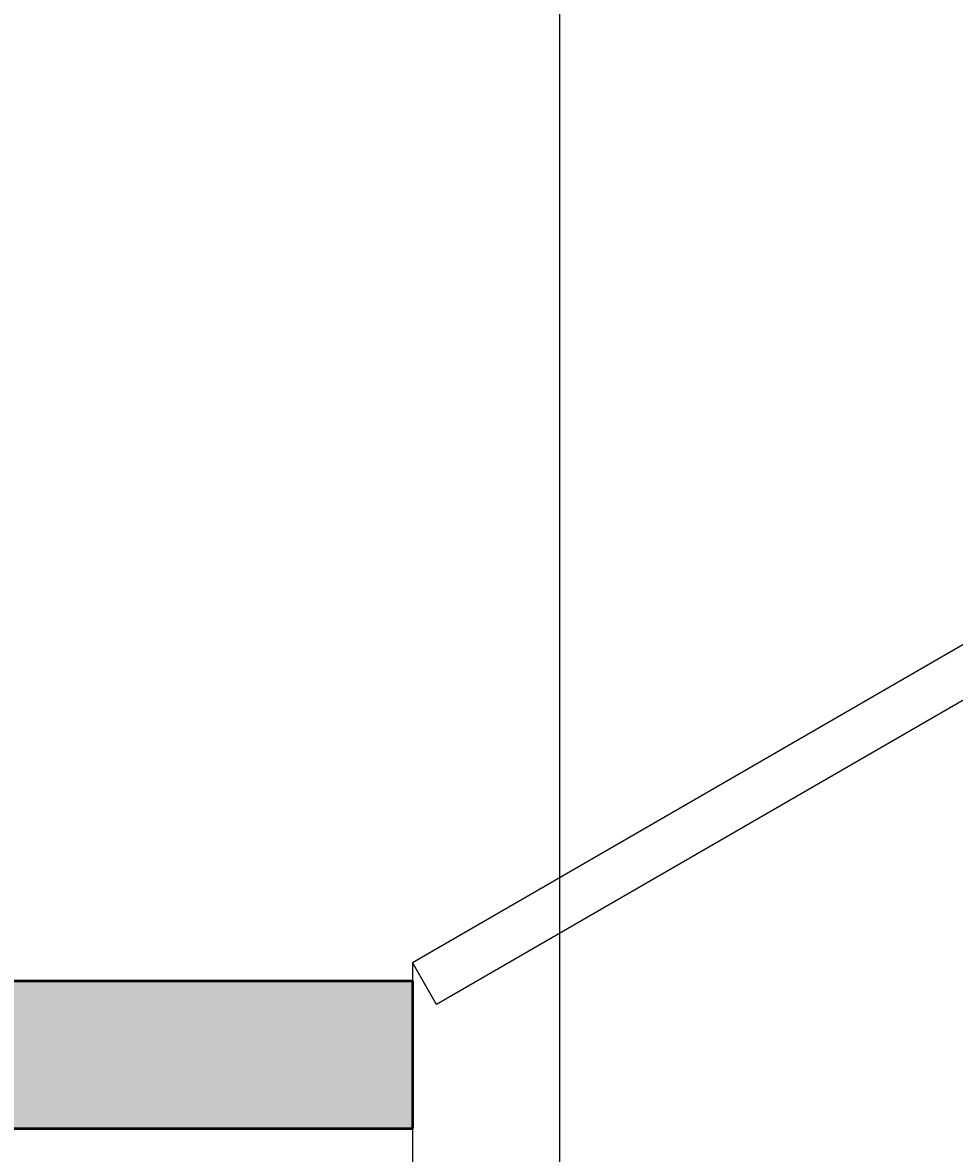
# Model space of a CAD drawing. Units: inches. Extents: x 2231 to 2461, y 2045 to 2455.
# Tile 55 of 95: x 2320 to 2346, y 2302 to 2333. Entities that reach past the tile are written whole.
import ezdxf

# ---------------------------------------------------------------- set-up
doc = ezdxf.new("R2010")
doc.units = ezdxf.units.IN
for name, color, linetype, lineweight in [('A-ANNO-DIMS', 2, 'Continuous', 18), ('A-DOOR', 3, 'Continuous', 25), ('A-WALL', 7, 'Continuous', 50)]:
    doc.layers.add(name, color=color, linetype=linetype, lineweight=lineweight)
doc.layers.add('A-WALL-PATT', color=18, linetype='Continuous', lineweight=13, true_color=0x000000)
doc.styles.get("Standard").update_dxf_attribs({"font": 'arial.ttf'})
doc.dimstyles.get("Standard").update_dxf_attribs({"dimtxt": 0.18, "dimasz": 0.18, "dimexe": 0.18, "dimexo": 0.0625, "dimgap": 0.09, "dimtad": 0, "dimtih": 1, "dimtoh": 1, "dimdec": 4, "dimzin": 0, "dimdsep": 46, "dimtxsty": 'Standard', "dimcen": 0.09, "dimadec": 0, "dimazin": 0, "dimtfac": 1, "dimtdec": 4, "dimtofl": 0, "dimtmove": 0, "dimatfit": 3, "dimfxl": 1, "dimtolj": 1, "dimtzin": 0, "dimarcsym": 0})

# ---------------------------------------------------------------- blocks, each defined once
blk = doc.blocks.new('*U3')
for p, q in [((0, 0), (0, -6)), ((40, 0), (40, -6))]:
    blk.add_line(p, q)
blk.add_lwpolyline([(0, 0), (34.641, 20), (35.516, 18.484), (0.875, -1.516)], close=True)
blk.add_arc((0, 0), 40, 0, 30)
blk = doc.blocks.new('*D50')
at = {"layer": 'A-ANNO-DIMS', "color": 0, "lineweight": -2, "transparency": 16777216}
for p, q in [((2304.794, 2182.895), (2304.794, 2454.645)), ((2304.974, 2454.465), (2319.575, 2454.465)), ((2334.614, 2454.465), (2320.012, 2454.465)), ((2334.794, 2182.895), (2334.794, 2454.645))]:
    blk.add_line(p, q, dxfattribs=at)
at = {"layer": 'A-ANNO-DIMS', "color": 0, "transparency": 16777216}
for points in [[(2304.974, 2454.495), (2304.974, 2454.435), (2304.794, 2454.465)], [(2334.614, 2454.495), (2334.614, 2454.435), (2334.794, 2454.465)]]:
    blk.add_solid(points, dxfattribs=at)
at = {"layer": 'Defpoints', "color": 0, "transparency": 16777216}
for p in [(2334.794, 2454.465), (2304.794, 2182.833), (2334.794, 2182.833)]:
    blk.add_point(p, dxfattribs=at)
at = {"layer": 'A-ANNO-DIMS', "color": 0, "transparency": 16777216, "insert": (2319.794, 2454.465), "char_height": 0.18, "attachment_point": 5}
blk.add_mtext('\\A1;30', dxfattribs=at)
blk = doc.blocks.new('*D51')
at = {"layer": 'A-ANNO-DIMS', "color": 0, "lineweight": -2, "transparency": 16777216}
for p, q in [((2258.794, 2306.77), (2258.794, 2044.803)), ((2330.794, 2306.77), (2330.794, 2044.803)), ((2258.974, 2044.983), (2294.576, 2044.983)), ((2330.614, 2044.983), (2295.011, 2044.983))]:
    blk.add_line(p, q, dxfattribs=at)
at = {"layer": 'A-ANNO-DIMS', "color": 0, "transparency": 16777216}
for points in [[(2258.974, 2045.013), (2258.974, 2044.953), (2258.794, 2044.983)], [(2330.614, 2045.013), (2330.614, 2044.953), (2330.794, 2044.983)]]:
    blk.add_solid(points, dxfattribs=at)
at = {"layer": 'Defpoints', "color": 0, "transparency": 16777216}
for p in [(2258.794, 2306.833), (2330.794, 2306.833), (2330.794, 2044.983)]:
    blk.add_point(p, dxfattribs=at)
at = {"layer": 'A-ANNO-DIMS', "color": 0, "transparency": 16777216, "insert": (2294.794, 2044.983), "char_height": 0.18, "attachment_point": 5}
blk.add_mtext('\\A1;72', dxfattribs=at)
blk = doc.blocks.new('*D52')
at = {"layer": 'A-ANNO-DIMS', "color": 0, "lineweight": -2, "transparency": 16777216}
for p, q in [((2330.794, 2306.77), (2330.794, 2044.803)), ((2360.794, 2306.77), (2360.794, 2044.803)), ((2330.974, 2044.983), (2345.575, 2044.983)), ((2360.614, 2044.983), (2346.012, 2044.983))]:
    blk.add_line(p, q, dxfattribs=at)
at = {"layer": 'A-ANNO-DIMS', "color": 0, "transparency": 16777216}
for points in [[(2330.974, 2045.013), (2330.974, 2044.953), (2330.794, 2044.983)], [(2360.614, 2045.013), (2360.614, 2044.953), (2360.794, 2044.983)]]:
    blk.add_solid(points, dxfattribs=at)
at = {"layer": 'Defpoints', "color": 0, "transparency": 16777216}
for p in [(2330.794, 2306.833), (2360.794, 2306.833), (2360.794, 2044.983)]:
    blk.add_point(p, dxfattribs=at)
at = {"layer": 'A-ANNO-DIMS', "color": 0, "transparency": 16777216, "insert": (2345.794, 2044.983), "char_height": 0.18, "attachment_point": 5}
blk.add_mtext('\\A1;30', dxfattribs=at)

msp = doc.modelspace()

# ---------------------------------------------------------------- hatches: boundary and pattern name
at = {"layer": 'A-WALL-PATT'}
h = msp.add_hatch(color=256, dxfattribs=at)
h.dxf.hatch_style = 1
h.paths.add_polyline_path([(2441.7935, 2269.1535), (2432.7935, 2269.1535), (2432.7935, 2186.8328), (2396.7935, 2186.8328), (2396.7935, 2286.8328), (2394.7935, 2286.8328), (2394.7935, 2186.8328), (2334.7935, 2186.8328), (2334.7935, 2182.8328), (2432.7935, 2182.8328), (2432.7935, 2072.8328), (2416.6639, 2072.8328), (2416.6639, 2063.8328), (2441.7935, 2063.8328)])
h.paths.add_polyline_path([(2368.6639, 2072.8328), (2367.04, 2072.8328), (2330.7942, 2072.8328), (2330.7397, 2063.8328), (2368.6639, 2063.8328)])
h.paths.add_polyline_path([(2300.7392, 2068.3328), (2300.7392, 2072.8328), (2298.7935, 2072.8328), (2294.7935, 2072.8328), (2258.7935, 2072.8328), (2258.7935, 2120.8328), (2294.7935, 2120.8328), (2298.7935, 2120.8328), (2298.7935, 2128.8328), (2294.7935, 2128.8328), (2294.7935, 2124.8328), (2258.7935, 2124.8328), (2258.7935, 2182.8328), (2294.7935, 2182.8328), (2294.7935, 2174.8328), (2298.7935, 2174.8328), (2298.7935, 2182.8328), (2304.7935, 2182.8328), (2304.7935, 2186.8328), (2258.7935, 2186.8328), (2258.7935, 2221.999), (2249.7935, 2221.999), (2249.7935, 2063.8328), (2300.7392, 2063.8328)])
h.paths.add_polyline_path([(2391.9338, 2435.8328), (2333.82, 2435.8328), (2333.82, 2426.8328), (2368.7935, 2426.8328), (2368.7935, 2374.9508), (2368.7935, 2370.8328), (2372.3935, 2370.8328), (2372.7935, 2370.8328), (2372.7935, 2426.8328), (2391.9338, 2426.8328)])
h.paths.add_polyline_path([(2441.7935, 2435.8328), (2415.9338, 2435.8328), (2415.9338, 2426.8328), (2432.7935, 2426.8328), (2432.7935, 2334.8328), (2372.7935, 2334.8328), (2372.7935, 2346.8328), (2368.7935, 2346.8328), (2368.7935, 2306.8328), (2360.7935, 2306.8328), (2360.7935, 2302.8328), (2368.7935, 2302.8328), (2372.7935, 2302.8328), (2372.7935, 2330.8328), (2432.7935, 2330.8328), (2432.7935, 2317.1535), (2441.7935, 2317.1535)])
h.paths.add_polyline_path([(2285.82, 2435.8328), (2249.7935, 2435.8328), (2249.7935, 2269.999), (2258.7935, 2269.999), (2258.7935, 2302.8328), (2318.8168, 2302.8328), (2330.7935, 2302.8328), (2330.7935, 2306.8328), (2258.7935, 2306.8328), (2258.7935, 2426.8328), (2285.82, 2426.8328)])

# ---------------------------------------------------------------- linework, layer by layer
at = {"layer": 'A-WALL'}
for p, q in [((2258.7935, 2306.8328), (2330.7935, 2306.8328)), ((2330.7935, 2306.8328), (2330.7935, 2302.8328)), ((2258.7935, 2302.8328), (2330.7935, 2302.8328))]:
    msp.add_line(p, q, dxfattribs=at)

# ---------------------------------------------------------------- block references
at = {"layer": 'A-DOOR', "xscale": 0.75, "yscale": 0.75, "zscale": 0.75}
msp.add_blockref('*U3', (2330.7935, 2307.3328), dxfattribs=at)

# ---------------------------------------------------------------- dimensions: what is measured, and where the dimension line sits
at = {"layer": 'A-ANNO-DIMS'}
for base, p1, p2, picture, middle in [((2334.7935, 2454.4653), (2304.7935, 2182.8328), (2334.7935, 2182.8328), '*D50', (2319.7935, 2454.4653)), ((2330.7935, 2044.9825), (2258.7935, 2306.8328), (2330.7935, 2306.8328), '*D51', (2294.7935, 2044.9825)), ((2360.7935, 2044.9825), (2330.7935, 2306.8328), (2360.7935, 2306.8328), '*D52', (2345.7935, 2044.9825))]:
    dim = msp.add_linear_dim(base=base, p1=p1, p2=p2, dimstyle='Standard', override={"dimdec": 0, "dimlfac": 1, "dimrnd": 0, "dimzin": 0, "dimdsep": 46, "dimlunit": 2}, dxfattribs=at)
    dim.commit()
    dim.dimension.update_dxf_attribs({"geometry": picture, "text_midpoint": middle})

doc.saveas('drawing.dxf')
